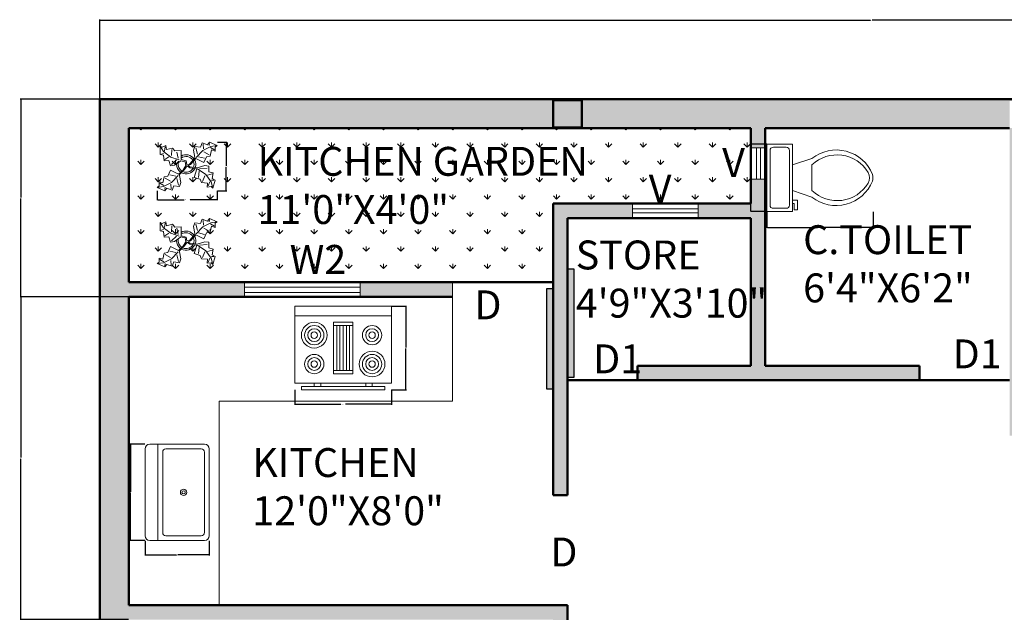
# Model space of a CAD drawing. Units: inches. Extents: x 1099 to 1629, y 1139 to 1548.
# Tile 2 of 3: x 1099 to 1405, y 1364 to 1548. Entities that reach past the tile are written whole.
import ezdxf

# ---------------------------------------------------------------- set-up
doc = ezdxf.new("R2010")
doc.units = ezdxf.units.IN
for name, color, linetype, lineweight in [('A-ANNO-DIMS', 2, 'Continuous', 18), ('A-ANNO-TEXT', 7, 'Continuous', 18), ('A-AREA-IDEN', 7, 'Continuous', 18), ('A-EQPM', 9, 'Continuous', 20), ('A-FLOR-FIXT', 9, 'Continuous', 20), ('A-FURN-FIXD', 2, 'Continuous', 18), ('A-WALL', 1, 'Continuous', 50), ('L-PLNT', 3, 'Continuous', 18), ('L-PLNT-PATT', 3, 'Continuous', 13)]:
    doc.layers.add(name, color=color, linetype=linetype, lineweight=lineweight)
for name, color, linetype, lineweight, true_color in [('A-COLS', 177, 'Continuous', 50, 0x293189), ('A-COLS-PATT', 177, 'Continuous', 13, 0x293189), ('A-DOOR', 30, 'Continuous', 25, 0xf26722), ('A-DOOR-PATT', 30, 'Continuous', 13, 0xf26722), ('A-GLAZ', 177, 'Continuous', 20, 0x293189), ('A-WALL-PATT', 244, 'Continuous', 13, 0x991b1e)]:
    doc.layers.add(name, color=color, linetype=linetype, lineweight=lineweight, true_color=true_color)
doc.styles.get("Standard").update_dxf_attribs({"font": 'arial.ttf'})
doc.dimstyles.get("Standard").update_dxf_attribs({"dimtxt": 0.18, "dimasz": 0.18, "dimexe": 0.18, "dimexo": 0.0625, "dimgap": 0.09, "dimtad": 0, "dimtih": 1, "dimtoh": 1, "dimdec": 4, "dimzin": 0, "dimdsep": 46, "dimtxsty": 'Standard', "dimcen": 0.09, "dimadec": 0, "dimazin": 0, "dimtfac": 1, "dimtdec": 4, "dimtofl": 0, "dimtmove": 0, "dimatfit": 3, "dimfxl": 1, "dimtolj": 1, "dimtzin": 0, "dimarcsym": 0})

# ---------------------------------------------------------------- blocks, each defined once
blk = doc.blocks.new('Toilet - top')
for p, q in [((9.5, -6), (9.5, -2)), ((-10, -8.5), (-8, -8.5)), ((-10, -9.5), (-10, -8.5)), ((-8, -8.5), (-8, -8)), ((-7, -8), (-7, -9.5)), ((-4, -8), (-6, -14)), ((4, -8), (6, -14)), ((-7, -9.5), (-10, -9.5)), ((4, -14), (-4, -14))]:
    blk.add_line(p, q)
blk.add_lwpolyline([(10.5, -8), (10.5, 0), (-10.5, 0), (-10.5, -8)], close=True)
for points in [[(-9.5, -2), (-9.5, -6)], [(8.5, -1), (-8.5, -1)], [(-8.5, -7), (8.5, -7)]]:
    blk.add_lwpolyline(points)
for centre, radius, start, end in [((-8.62, -1.88), 0.884, 81.8699, 188.1301), ((8.62, -1.88), 0.884, 351.8699, 98.1301), ((-8.62, -6.12), 0.884, 171.8699, 278.1301), ((8.62, -6.12), 0.884, 261.8699, 8.1301), ((3.52, -21.58), 12.17, 141.4691, 247.9714), ((4.2, -21.82), 11.33, 136.3677, 238.9468), ((-3.52, -21.58), 12.17, 292.0284, 38.5307), ((-4.2, -21.82), 11.33, 301.053, 43.6321), ((0, -27.88), 4, 245.7318, 294.2682), ((0, -29), 4, 254.8605, 285.1395)]:
    blk.add_arc(centre, radius, start, end)
blk = doc.blocks.new('Range-Oven - 30 in top')
for p, q in [((0, -3), (30, -3)), ((12, -6), (18, -6)), ((13, -20), (13, -6)), ((14, -6), (14, -20)), ((15, -20), (15, -6)), ((16, -6), (16, -20)), ((17, -20), (17, -6)), ((18, -20), (12, -20)), ((6, -24), (6, -25)), ((8, -25), (8, -24)), ((22, -25), (22, -24)), ((24, -24), (24, -25))]:
    blk.add_line(p, q)
for points in [[(0, -24), (0, 0), (30, 0), (30, -24)], [(12, -21), (12, -5), (18, -5), (18, -21)], [(2, -26), (2, -25), (28, -25), (28, -26)]]:
    blk.add_lwpolyline(points, close=True)
for centre, radius in [((6, -9), 4), ((6, -9), 3), ((24, -9), 3), ((6, -9), 2), ((6, -9), 1), ((24, -9), 2), ((24, -9), 1), ((6, -18), 3), ((24, -18), 4), ((24, -18), 3), ((6, -18), 2), ((6, -18), 1), ((24, -18), 2), ((24, -18), 1)]:
    blk.add_circle(centre, radius)
blk = doc.blocks.new('Sink-single - 30 in top')
blk.add_line((-15, -3.999996), (15, -3.999996))
for points in [[(-13.5, 0), (13.5, 0)], [(-15, -18.499996), (-15, -1.5)], [(15, -1.5), (15, -18.499996)], [(-12.5, -5.499996), (12.5, -5.499996)], [(-13.5, -17.499996), (-13.5, -6.499996)], [(13.5, -6.499996), (13.5, -17.499996)], [(13.5, -19.999996), (-13.5, -19.999996)], [(12.5, -18.499996), (-12.5, -18.499996)]]:
    blk.add_lwpolyline(points)
for radius in [1, 0.5]:
    blk.add_circle((0, -11.999996), radius)
for centre, radius, start, end in [((-13.5, -1.5), 1.5, 90, 180), ((13.5, -1.5), 1.5, 0, 90), ((-12.5, -6.499996), 1, 90, 180), ((12.5, -6.499996), 1, 0, 90), ((-12.5, -17.499996), 1, 180, 270), ((12.5, -17.499996), 1, 270, 0), ((-13.5, -18.499996), 1.5, 180, 270), ((13.5, -18.499996), 1.5, 270, 0)]:
    blk.add_arc(centre, radius, start, end)
blk = doc.blocks.new('Plant - Rubber or Philodendron')
for p, q in [((8.8871, 10.7908), (9.9809, 13.4933)), ((9.9809, 13.4933), (13.3837, 12.301)), ((10.5828, 12.6946), (10.8893, 9.7953)), ((13.3837, 12.301), (14.68, 13.9039)), ((14.5816, 13.2037), (14.3848, 11.8033)), ((14.68, 13.9039), (19.3848, 11.8146)), ((-16.2005, 11.4774), (-13.9899, 8.1064)), ((-16.2005, 11.4774), (-14.8639, 10.7964)), ((-16.0159, 6.3329), (-16.2005, 11.4774)), ((-14.0069, 5.8704), (-16.0159, 6.3329)), ((-15.3434, 6.5514), (-13.9984, 6.9884)), ((-14.8639, 10.7964), (-12.6195, 11.8975)), ((-13.9899, 8.1064), (-9.5434, 4.7185)), ((-13.3174, 8.325), (-13.0735, 11.0065)), ((-12.6195, 11.8975), (-12.1909, 9.4345)), ((-12.1909, 9.4345), (-8.3829, 10.3)), ((-8.8369, 9.409), (-9.0894, 5.6095)), ((-8.3829, 10.3), (-7.0549, 8.501)), ((-7.0549, 8.501), (-3.0284, 8.6941)), ((-4.8529, 4.012), (-5.7184, 7.82)), ((-3.0284, 8.6941), (-3.0709, 3.1041)), ((4.6914, 8.8812), (5.3859, 11.2828)), ((4.6914, 8.8812), (5.5014, 4.4831)), ((5.3859, 11.2828), (8.8871, 10.7908)), ((5.9878, 10.4842), (7.1971, 6.3869)), ((10.3916, 8.7942), (6.2847, 4.4028)), ((15.3859, 11.3055), (10.3916, 8.7942)), ((14.2977, 6.1031), (10.9934, 7.9956)), ((15.7909, 9.1065), (14.8995, 5.3044)), ((15.2875, 10.6053), (17.5907, 9.2105)), ((19.3848, 11.8146), (15.3859, 11.3055)), ((18.1925, 8.4119), (15.7909, 9.1065)), ((19.3848, 11.8146), (18.1868, 10.9119)), ((18.1868, 10.9119), (18.1925, 8.4119)), ((-13.5868, 2.2894), (-14.0069, 5.8704)), ((-10.6784, 2.491), (-13.5868, 2.2894)), ((-13.1329, 3.1804), (-10.6614, 4.727)), ((-9.5858, -0.8715), (-10.6784, 2.491)), ((-9.5434, 4.7185), (-4.1917, 2.9888)), ((-9.1318, 0.0195), (-5.9793, 2.9025)), ((-7.1228, -0.443), (-3.5248, 2.2131)), ((-3.5248, 2.2131), (-3.3011, 2.4355)), ((-3.3011, 2.4355), (-0.5306, 1.7947)), ((-3.0709, 3.1041), (0.0797, 2.3163)), ((-0.5306, 1.7947), (-0.2255, -0.5527)), ((-0.5306, 1.7947), (-0.5306, 1.7947)), ((0.0797, 2.3163), (0.4866, -0.031)), ((0.4866, -0.031), (2.1141, 0.2298)), ((2.1141, 0.2298), (5.4346, 3.9146)), ((6.1032, 3.6844), (2.8262, -0.031)), ((5.4346, 3.9146), (5.5014, 4.4831)), ((11.1089, 1.1958), (6.1032, 3.6844)), ((7.7005, 4.8881), (11.5025, 3.9967)), ((12.7005, 4.8994), (11.1089, 1.1958)), ((14.8995, 5.3044), (12.7005, 4.8994)), ((-11.3237, -7.2629), (-9.7321, -3.5593)), ((-9.7321, -3.5593), (-4.7264, -6.0479)), ((-7.1228, -0.443), (-9.5858, -0.8715)), ((-2.019, -3.6148), (-4.7264, -6.0479)), ((-4.0579, -6.2781), (-0.9375, -3.1608)), ((-2.019, -3.6148), (-0.2255, -0.5527)), ((-0.9375, -3.1608), (0.5883, -0.8135)), ((0.5883, -0.8135), (2.2447, -2.0916)), ((2.8262, -0.031), (1.3003, -0.5527)), ((1.3003, -0.5527), (2.4193, -1.4655)), ((2.2447, -2.0916), (6.7108, -2.6626)), ((2.4193, -1.4655), (6.895, -2.1175)), ((4.943, -7.9659), (6.7108, -2.6626)), ((11.6605, -0.5413), (6.895, -2.1175)), ((12.3677, -6.1981), (7.219, -2.6772)), ((8.125, -4.0768), (7.7715, -7.9659)), ((8.3544, -2.7453), (13.1973, -2.1704)), ((11.6605, -0.5413), (14.1354, -0.8948)), ((16.2567, -5.8446), (13.4283, -6.5517)), ((14.1354, -0.8948), (14.1354, -4.4304)), ((14.1354, -4.4304), (16.9638, -5.1375)), ((16.9638, -5.1375), (16.2567, -8.673)), ((-16.8157, -10.7754), (-14.4141, -11.4699)), ((-16.8101, -13.2754), (-16.8157, -10.7754)), ((-13.9107, -12.9688), (-16.2139, -11.574)), ((-14.4141, -11.4699), (-13.5228, -7.6679)), ((-14.0091, -13.669), (-9.0148, -11.1577)), ((-13.5228, -7.6679), (-11.3237, -7.2629)), ((-12.921, -8.4665), (-9.6166, -10.359)), ((-6.3237, -7.2516), (-10.1257, -6.3602)), ((-9.206, -15.0581), (-9.5126, -12.1588)), ((-9.0148, -11.1577), (-4.9047, -6.8122)), ((-4.611, -12.8477), (-5.8203, -8.7504)), ((-4.1246, -6.8466), (-4.0579, -6.2781)), ((-3.3146, -11.2447), (-4.1246, -6.8466)), ((-3.3146, -11.2447), (-4.0092, -13.6463)), ((8.8321, -9.0266), (4.943, -7.9659)), ((9.5392, -11.1479), (8.8321, -9.0266)), ((13.4283, -11.5015), (9.5392, -11.1479)), ((10.2463, -10.4408), (11.6605, -6.9053)), ((15.5496, -10.7943), (12.3677, -6.1981)), ((13.0748, -13.9763), (13.4283, -11.5015)), ((14.8425, -10.7943), (13.7819, -13.2692)), ((16.6103, -14.6834), (15.5496, -10.7943)), ((17.3174, -9.7337), (15.9032, -9.7337)), ((16.2567, -8.673), (18.0245, -9.7337)), ((18.0245, -9.7337), (16.6103, -14.6834)), ((-18.008, -14.1781), (-16.8101, -13.2754)), ((-18.008, -14.1781), (-14.0091, -13.669)), ((-13.3032, -16.2674), (-18.008, -14.1781)), ((-12.0069, -14.6645), (-13.3032, -16.2674)), ((-13.2048, -15.5672), (-13.008, -14.1668)), ((-8.6042, -15.8568), (-12.0069, -14.6645)), ((-7.5103, -13.1543), (-8.6042, -15.8568)), ((-4.0092, -13.6463), (-7.5103, -13.1543)), ((15.5496, -13.6228), (13.0748, -13.9763)), ((16.6103, -14.6834), (15.5496, -13.6228))]:
    blk.add_line(p, q)
for centre, radius, start, end in [((0, 0), 6.1275, 34.37569, 120.1028), ((0.0308, 0.1664), 6, 178.6147, 235.1169), ((0.0308, 0.1664), 5, 168.1647, 238.6725), ((-0.0601, -0.2075), 5.2461, 33.82192, 124.9414), ((-0.2664, 0.1682), 5.2775, 338.4094, 20.03007), ((-0.098, 0.1364), 6.1288, 341.2017, 26.09184), ((-0.0234, 0.3825), 6.1492, 242.5812, 331.2714), ((-0.1102, 0.4886), 5.2883, 247.3711, 327.472)]:
    blk.add_arc(centre, radius, start, end)
blk = doc.blocks.new('*D11')
at = {"layer": 'A-ANNO-DIMS', "color": 0, "lineweight": -2, "transparency": 16777216}
for p, q in [((1331.62, 1488.62), (1331.62, 1483.55)), ((1364.67, 1488.62), (1364.67, 1483.55)), ((1331.8, 1483.73), (1347.37, 1483.73)), ((1364.49, 1483.73), (1348.92, 1483.73))]:
    blk.add_line(p, q, dxfattribs=at)
at = {"layer": 'A-ANNO-DIMS', "color": 0, "lineweight": 100, "transparency": 16777216}
for points in [[(1331.8, 1483.76), (1331.8, 1483.7), (1331.62, 1483.73)], [(1364.49, 1483.76), (1364.49, 1483.7), (1364.67, 1483.73)]]:
    blk.add_solid(points, dxfattribs=at)
at = {"layer": 'Defpoints', "color": 0, "lineweight": 100, "transparency": 16777216}
for p in [(1331.62, 1488.69), (1364.67, 1488.69), (1331.62, 1483.73)]:
    blk.add_point(p, dxfattribs=at)
at = {"layer": 'A-ANNO-DIMS', "color": 0, "transparency": 16777216, "insert": (1348.14, 1483.73), "char_height": 0.18, "attachment_point": 5}
blk.add_mtext('\\A1;WC 33 TYP.', dxfattribs=at)
blk = doc.blocks.new('*D12')
at = {"layer": 'A-ANNO-DIMS', "color": 0, "lineweight": -2, "transparency": 16777216}
for p, q in [((1331.56, 1509.69), (1326.48, 1509.69)), ((1326.66, 1509.51), (1326.66, 1499.37)), ((1326.66, 1488.87), (1326.66, 1499)), ((1331.56, 1488.69), (1326.48, 1488.69))]:
    blk.add_line(p, q, dxfattribs=at)
at = {"layer": 'A-ANNO-DIMS', "color": 0, "lineweight": 100, "transparency": 16777216}
for points in [[(1326.63, 1509.51), (1326.69, 1509.51), (1326.66, 1509.69)], [(1326.63, 1488.87), (1326.69, 1488.87), (1326.66, 1488.69)]]:
    blk.add_solid(points, dxfattribs=at)
at = {"layer": 'Defpoints', "color": 0, "lineweight": 100, "transparency": 16777216}
for p in [(1326.66, 1509.69), (1331.62, 1509.69), (1331.62, 1488.69)]:
    blk.add_point(p, dxfattribs=at)
at = {"layer": 'A-ANNO-DIMS', "color": 0, "transparency": 16777216, "insert": (1326.66, 1499.19), "char_height": 0.18, "attachment_point": 5}
blk.add_mtext('\\A1;21 TYP.', dxfattribs=at)
blk = doc.blocks.new('*D15')
at = {"layer": 'A-ANNO-DIMS', "color": 0, "lineweight": -2, "transparency": 16777216}
for p, q in [((1184.82, 1433.12), (1184.82, 1428.5)), ((1214.82, 1433.12), (1214.82, 1428.5)), ((1185, 1428.68), (1199.12, 1428.68)), ((1214.64, 1428.68), (1200.51, 1428.68))]:
    blk.add_line(p, q, dxfattribs=at)
at = {"layer": 'A-ANNO-DIMS', "color": 0, "lineweight": 100, "transparency": 16777216}
for points in [[(1185, 1428.71), (1185, 1428.65), (1184.82, 1428.68)], [(1214.64, 1428.71), (1214.64, 1428.65), (1214.82, 1428.68)]]:
    blk.add_solid(points, dxfattribs=at)
at = {"layer": 'Defpoints', "color": 0, "lineweight": 100, "transparency": 16777216}
for p in [(1184.82, 1433.18), (1214.82, 1433.18), (1214.82, 1428.68)]:
    blk.add_point(p, dxfattribs=at)
at = {"layer": 'A-ANNO-DIMS', "color": 0, "transparency": 16777216, "insert": (1199.82, 1428.68), "char_height": 0.18, "attachment_point": 5}
blk.add_mtext('\\A1;RANGE 30', dxfattribs=at)
blk = doc.blocks.new('*D16')
at = {"layer": 'A-ANNO-DIMS', "color": 0, "lineweight": -2, "transparency": 16777216}
for p, q in [((1214.88, 1459.18), (1219.5, 1459.18)), ((1219.32, 1459), (1219.32, 1446.36)), ((1219.32, 1433.36), (1219.32, 1446)), ((1214.88, 1433.18), (1219.5, 1433.18))]:
    blk.add_line(p, q, dxfattribs=at)
at = {"layer": 'A-ANNO-DIMS', "color": 0, "lineweight": 100, "transparency": 16777216}
for points in [[(1219.29, 1459), (1219.35, 1459), (1219.32, 1459.18)], [(1219.29, 1433.36), (1219.35, 1433.36), (1219.32, 1433.18)]]:
    blk.add_solid(points, dxfattribs=at)
at = {"layer": 'Defpoints', "color": 0, "lineweight": 100, "transparency": 16777216}
for p in [(1214.82, 1459.18), (1219.32, 1459.18), (1214.82, 1433.18)]:
    blk.add_point(p, dxfattribs=at)
at = {"layer": 'A-ANNO-DIMS', "color": 0, "transparency": 16777216, "insert": (1219.32, 1446.18), "char_height": 0.18, "attachment_point": 5}
blk.add_mtext('\\A1;26', dxfattribs=at)
blk = doc.blocks.new('*D17')
at = {"layer": 'A-ANNO-DIMS', "color": 0, "lineweight": -2, "transparency": 16777216}
for p, q in [((1138.11, 1416.24), (1133.5, 1416.24)), ((1133.68, 1416.06), (1133.68, 1401.42)), ((1133.68, 1386.42), (1133.68, 1401.06)), ((1138.11, 1386.24), (1133.5, 1386.24))]:
    blk.add_line(p, q, dxfattribs=at)
at = {"layer": 'A-ANNO-DIMS', "color": 0, "lineweight": 100, "transparency": 16777216}
for points in [[(1133.65, 1416.06), (1133.71, 1416.06), (1133.68, 1416.24)], [(1133.65, 1386.42), (1133.71, 1386.42), (1133.68, 1386.24)]]:
    blk.add_solid(points, dxfattribs=at)
at = {"layer": 'Defpoints', "color": 0, "lineweight": 100, "transparency": 16777216}
for p in [(1133.68, 1416.24), (1138.18, 1416.24), (1138.18, 1386.24)]:
    blk.add_point(p, dxfattribs=at)
at = {"layer": 'A-ANNO-DIMS', "color": 0, "transparency": 16777216, "insert": (1133.68, 1401.24), "char_height": 0.18, "attachment_point": 5}
blk.add_mtext('\\A1;SINK 30', dxfattribs=at)
blk = doc.blocks.new('*D18')
at = {"layer": 'A-ANNO-DIMS', "color": 0, "lineweight": -2, "transparency": 16777216}
for p, q in [((1138.18, 1386.18), (1138.18, 1381.56)), ((1158.18, 1386.18), (1158.18, 1381.56)), ((1138.36, 1381.74), (1147.96, 1381.74)), ((1158, 1381.74), (1148.4, 1381.74))]:
    blk.add_line(p, q, dxfattribs=at)
at = {"layer": 'A-ANNO-DIMS', "color": 0, "lineweight": 100, "transparency": 16777216}
for points in [[(1138.36, 1381.77), (1138.36, 1381.71), (1138.18, 1381.74)], [(1158, 1381.77), (1158, 1381.71), (1158.18, 1381.74)]]:
    blk.add_solid(points, dxfattribs=at)
at = {"layer": 'Defpoints', "color": 0, "lineweight": 100, "transparency": 16777216}
for p in [(1138.18, 1386.24), (1158.18, 1386.24), (1138.18, 1381.74)]:
    blk.add_point(p, dxfattribs=at)
at = {"layer": 'A-ANNO-DIMS', "color": 0, "transparency": 16777216, "insert": (1148.18, 1381.74), "char_height": 0.18, "attachment_point": 5}
blk.add_mtext('\\A1;20', dxfattribs=at)
blk = doc.blocks.new('*D23')
at = {"layer": 'A-ANNO-DIMS', "color": 0, "lineweight": -2, "transparency": 16777216}
for p, q in [((1141.94, 1495.09), (1141.94, 1492.17)), ((1160.64, 1495.09), (1160.64, 1492.17)), ((1142.12, 1492.35), (1150.32, 1492.35)), ((1160.46, 1492.35), (1152.25, 1492.35))]:
    blk.add_line(p, q, dxfattribs=at)
at = {"layer": 'A-ANNO-DIMS', "color": 0, "lineweight": 100, "transparency": 16777216}
for points in [[(1142.12, 1492.38), (1142.12, 1492.32), (1141.94, 1492.35)], [(1160.46, 1492.38), (1160.46, 1492.32), (1160.64, 1492.35)]]:
    blk.add_solid(points, dxfattribs=at)
at = {"layer": 'Defpoints', "color": 0, "lineweight": 100, "transparency": 16777216}
for p in [(1141.94, 1495.16), (1160.64, 1495.16), (1160.64, 1492.35)]:
    blk.add_point(p, dxfattribs=at)
at = {"layer": 'A-ANNO-DIMS', "color": 0, "transparency": 16777216, "insert": (1151.29, 1492.35), "char_height": 0.18, "attachment_point": 5}
blk.add_mtext('\\A1;PLANT 19 TYP.', dxfattribs=at)
blk = doc.blocks.new('*D24')
at = {"layer": 'A-ANNO-DIMS', "color": 0, "lineweight": -2, "transparency": 16777216}
for p, q in [((1160.7, 1510.24), (1163.62, 1510.24)), ((1163.44, 1510.06), (1163.44, 1502.88)), ((1163.44, 1495.34), (1163.44, 1502.52)), ((1160.7, 1495.16), (1163.62, 1495.16))]:
    blk.add_line(p, q, dxfattribs=at)
at = {"layer": 'A-ANNO-DIMS', "color": 0, "lineweight": 100, "transparency": 16777216}
for points in [[(1163.41, 1510.06), (1163.47, 1510.06), (1163.44, 1510.24)], [(1163.41, 1495.34), (1163.47, 1495.34), (1163.44, 1495.16)]]:
    blk.add_solid(points, dxfattribs=at)
at = {"layer": 'Defpoints', "color": 0, "lineweight": 100, "transparency": 16777216}
for p in [(1160.64, 1510.24), (1163.44, 1510.24), (1160.64, 1495.16)]:
    blk.add_point(p, dxfattribs=at)
at = {"layer": 'A-ANNO-DIMS', "color": 0, "transparency": 16777216, "insert": (1163.44, 1502.7), "char_height": 0.18, "attachment_point": 5}
blk.add_mtext('\\A1;15 TYP.', dxfattribs=at)
blk = doc.blocks.new('*D25')
at = {"layer": 'A-ANNO-DIMS', "color": 0, "lineweight": -2, "transparency": 16777216}
for p, q in [((1124.1, 1523.69), (1124.1, 1548.41)), ((1124.28, 1548.23), (1363.81, 1548.23)), ((1603.92, 1548.23), (1364.39, 1548.23)), ((1604.1, 1523.69), (1604.1, 1548.41))]:
    blk.add_line(p, q, dxfattribs=at)
at = {"layer": 'A-ANNO-DIMS', "color": 0, "lineweight": 100, "transparency": 16777216}
for points in [[(1124.28, 1548.26), (1124.28, 1548.2), (1124.1, 1548.23)], [(1603.92, 1548.26), (1603.92, 1548.2), (1604.1, 1548.23)]]:
    blk.add_solid(points, dxfattribs=at)
at = {"layer": 'Defpoints', "color": 0, "lineweight": 100, "transparency": 16777216}
for p in [(1604.1, 1548.23), (1124.1, 1523.63), (1604.1, 1523.63)]:
    blk.add_point(p, dxfattribs=at)
at = {"layer": 'A-ANNO-DIMS', "color": 0, "transparency": 16777216, "insert": (1364.1, 1548.23), "char_height": 0.18, "attachment_point": 5}
blk.add_mtext('\\A1;480', dxfattribs=at)
blk = doc.blocks.new('*D36')
at = {"layer": 'A-ANNO-DIMS', "color": 0, "lineweight": -2, "transparency": 16777216}
for p, q in [((1133.04, 1462.13), (1099.32, 1462.13)), ((1099.5, 1461.95), (1099.5, 1412.06)), ((1099.5, 1361.81), (1099.5, 1411.7)), ((1133.04, 1361.63), (1099.32, 1361.63))]:
    blk.add_line(p, q, dxfattribs=at)
at = {"layer": 'A-ANNO-DIMS', "color": 0, "lineweight": 100, "transparency": 16777216}
for points in [[(1099.47, 1461.95), (1099.53, 1461.95), (1099.5, 1462.13)], [(1099.47, 1361.81), (1099.53, 1361.81), (1099.5, 1361.63)]]:
    blk.add_solid(points, dxfattribs=at)
at = {"layer": 'Defpoints', "color": 0, "lineweight": 100, "transparency": 16777216}
for p in [(1099.5, 1462.13), (1133.1, 1462.13), (1133.1, 1361.63)]:
    blk.add_point(p, dxfattribs=at)
at = {"layer": 'A-ANNO-DIMS', "color": 0, "transparency": 16777216, "insert": (1099.5, 1411.88), "char_height": 0.18, "attachment_point": 5}
blk.add_mtext('\\A1;100.5', dxfattribs=at)
blk = doc.blocks.new('*D37')
at = {"layer": 'A-ANNO-DIMS', "color": 0, "lineweight": -2, "transparency": 16777216}
for p, q in [((1124.04, 1523.63), (1099.32, 1523.63)), ((1099.5, 1523.45), (1099.5, 1493.06)), ((1099.5, 1462.31), (1099.5, 1492.7)), ((1133.04, 1462.13), (1099.32, 1462.13))]:
    blk.add_line(p, q, dxfattribs=at)
at = {"layer": 'A-ANNO-DIMS', "color": 0, "lineweight": 100, "transparency": 16777216}
for points in [[(1099.47, 1523.45), (1099.53, 1523.45), (1099.5, 1523.63)], [(1099.47, 1462.31), (1099.53, 1462.31), (1099.5, 1462.13)]]:
    blk.add_solid(points, dxfattribs=at)
at = {"layer": 'Defpoints', "color": 0, "lineweight": 100, "transparency": 16777216}
for p in [(1099.5, 1523.63), (1124.1, 1523.63), (1133.1, 1462.13)]:
    blk.add_point(p, dxfattribs=at)
at = {"layer": 'A-ANNO-DIMS', "color": 0, "transparency": 16777216, "insert": (1099.5, 1492.88), "char_height": 0.18, "attachment_point": 5}
blk.add_mtext('\\A1;61.5', dxfattribs=at)

msp = doc.modelspace()

# ---------------------------------------------------------------- hatches: boundary and pattern name
at = {"layer": 'A-COLS-PATT'}
h = msp.add_hatch(color=256, dxfattribs=at)
h.dxf.hatch_style = 1
h.paths.add_polyline_path([(1265.099, 1514.872), (1274.099, 1514.872), (1274.099, 1523.316), (1265.099, 1523.316)])
at = {"layer": 'A-DOOR-PATT'}
h = msp.add_hatch(color=256, dxfattribs=at)
h.dxf.hatch_style = 1
h.paths.add_polyline_path([(1265.099, 1464.652), (1263.099, 1464.652), (1263.099, 1433.449), (1265.099, 1433.449)])
h.paths.add_polyline_path([(1271.599, 1470.878), (1269.599, 1470.878), (1269.599, 1437.014), (1271.599, 1437.014)])
at = {"layer": 'A-WALL-PATT'}
h = msp.add_hatch(color=256, dxfattribs=at)
h.dxf.hatch_style = 1
h.paths.add_polyline_path([(1407.099, 1523.072), (1416.099, 1523.072), (1416.099, 1514.628), (1595.099, 1514.628), (1595.099, 1523.072), (1604.099, 1523.072), (1604.099, 1523.628), (1124.099, 1523.628), (1124.099, 1172.072), (1133.099, 1172.072), (1133.099, 1361.628), (1265.099, 1361.628), (1265.099, 1301.628), (1269.599, 1301.628), (1269.599, 1366.128), (1133.099, 1366.128), (1133.099, 1462.128), (1169.127, 1462.128), (1169.127, 1466.628), (1133.099, 1466.628), (1133.099, 1514.628), (1265.099, 1514.628), (1265.099, 1514.872), (1265.099, 1523.316), (1274.099, 1523.316), (1274.099, 1514.628), (1326.599, 1514.628), (1326.599, 1508.465), (1331.099, 1508.465), (1331.099, 1514.628), (1407.099, 1514.628)])
h.paths.add_polyline_path([(1604.099, 1514.628), (1595.099, 1514.628), (1595.099, 1384.628), (1595.099, 1380.128), (1595.099, 1323.878), (1535.099, 1323.878), (1535.099, 1321.628), (1595.099, 1321.628), (1595.099, 1172.628), (1539.988, 1172.628), (1539.988, 1163.628), (1594.904, 1163.628), (1594.904, 1172.072), (1604.099, 1172.072)])
h.paths.add_polyline_path([(1461.599, 1380.128), (1530.599, 1380.128), (1530.599, 1363.564), (1535.099, 1363.564), (1535.099, 1380.128), (1535.099, 1384.628), (1416.099, 1384.628), (1416.099, 1380.128), (1457.099, 1380.128), (1457.099, 1326.128), (1457.099, 1321.628), (1504.951, 1321.628), (1504.951, 1326.128), (1461.599, 1326.128)], flags=17)
h.paths.add_polyline_path([(1535.099, 1346.252), (1530.599, 1346.252), (1530.599, 1326.128), (1530.599, 1321.628), (1535.099, 1321.628), (1535.099, 1323.878), (1535.099, 1326.128)], flags=16)
h.paths.add_polyline_path([(1269.599, 1301.628), (1265.099, 1301.628), (1260.599, 1301.628), (1260.599, 1214.628), (1260.599, 1205.628), (1265.099, 1205.628), (1269.599, 1205.628), (1269.599, 1214.628)], flags=17)
h.paths.add_polyline_path([(1411.599, 1262.279), (1451.001, 1262.279), (1451.001, 1266.779), (1411.599, 1266.779), (1411.599, 1342.184), (1407.099, 1342.184), (1407.099, 1214.628), (1386.727, 1214.628), (1386.727, 1205.628), (1407.099, 1205.628), (1407.099, 1163.628), (1491.988, 1163.628), (1491.988, 1172.628), (1411.599, 1172.628)])
h.paths.add_polyline_path([(1315.906, 1214.628), (1300.958, 1214.628), (1300.958, 1205.628), (1315.906, 1205.628)], flags=17)
h = msp.add_hatch(color=256, dxfattribs=at)
h.dxf.hatch_style = 1
h.paths.add_polyline_path([(1233.806, 1466.628), (1205.127, 1466.628), (1205.127, 1462.128), (1233.806, 1462.128)])
h.paths.add_polyline_path([(1269.599, 1486.628), (1289.77, 1486.628), (1289.77, 1491.128), (1269.599, 1491.128), (1265.099, 1491.128), (1265.099, 1400.307), (1269.599, 1400.307)])
h.paths.add_polyline_path([(1379.104, 1440.628), (1331.099, 1440.628), (1331.099, 1498.77), (1326.599, 1498.77), (1326.599, 1491.128), (1310.198, 1491.128), (1310.198, 1486.628), (1326.599, 1486.628), (1326.599, 1440.628), (1291.317, 1440.628), (1291.317, 1436.128), (1379.104, 1436.128)])
h.paths.add_polyline_path([(1416.099, 1514.628), (1407.099, 1514.628), (1407.099, 1418.838), (1411.599, 1418.838), (1438.846, 1418.838), (1438.846, 1423.338), (1416.099, 1423.338)])
at = {"layer": 'L-PLNT-PATT'}
h = msp.add_hatch(dxfattribs=at)
h.set_pattern_fill('GRASS', color=256, scale=0.3)
h.paths.add_polyline_path([(1265.099, 1491.128), (1269.599, 1491.128), (1326.599, 1491.128), (1326.599, 1514.628), (1133.099, 1514.628), (1133.099, 1466.628), (1265.099, 1466.628)])

# ---------------------------------------------------------------- linework, layer by layer
at = {"layer": 'A-COLS'}
msp.add_lwpolyline([(1265.099, 1514.872), (1274.099, 1514.872), (1274.099, 1523.316), (1265.099, 1523.316)], close=True, dxfattribs=at)
at = {"layer": 'A-DOOR'}
for p, q in [((1269.599, 1470.878), (1271.599, 1470.878)), ((1271.599, 1470.878), (1271.599, 1437.014)), ((1265.099, 1464.652), (1263.099, 1464.652)), ((1263.099, 1464.652), (1263.099, 1433.449)), ((1271.599, 1437.014), (1269.599, 1437.014)), ((1263.099, 1433.449), (1265.099, 1433.449))]:
    msp.add_line(p, q, dxfattribs=at)
at = {"layer": 'A-FURN-FIXD'}
for p, q in [((1233.806, 1466.628), (1233.806, 1438.761)), ((1233.806, 1438.761), (1233.806, 1429.661)), ((1161.284, 1429.661), (1161.284, 1366.128)), ((1233.806, 1429.661), (1161.284, 1429.661))]:
    msp.add_line(p, q, dxfattribs=at)
at = {"layer": 'A-GLAZ'}
for p, q in [((1331.099, 1508.465), (1326.599, 1508.465)), ((1328.406, 1508.465), (1328.406, 1498.77)), ((1329.664, 1508.465), (1329.664, 1498.77)), ((1331.099, 1498.77), (1326.599, 1498.77)), ((1289.77, 1491.128), (1289.77, 1486.628)), ((1310.198, 1489.495), (1289.77, 1489.495)), ((1310.198, 1491.128), (1310.198, 1486.628)), ((1310.198, 1488.239), (1289.77, 1488.239)), ((1169.127, 1466.628), (1169.127, 1462.128)), ((1169.127, 1465.16), (1205.127, 1465.16)), ((1205.127, 1466.628), (1205.127, 1462.128)), ((1169.127, 1463.462), (1205.127, 1463.462))]:
    msp.add_line(p, q, dxfattribs=at)
at = {"layer": 'A-WALL'}
for p, q in [((1604.099, 1523.628), (1124.099, 1523.628)), ((1124.099, 1523.628), (1124.099, 1163.628)), ((1133.099, 1514.628), (1133.099, 1466.628)), ((1265.099, 1514.628), (1133.099, 1514.628)), ((1326.599, 1514.628), (1133.099, 1514.628)), ((1326.599, 1514.628), (1326.599, 1491.128)), ((1407.099, 1514.628), (1331.099, 1514.628)), ((1331.099, 1514.628), (1331.099, 1440.628)), ((1265.099, 1491.128), (1265.099, 1400.307)), ((1269.599, 1491.128), (1265.099, 1491.128)), ((1326.599, 1491.128), (1269.599, 1491.128)), ((1326.599, 1486.628), (1269.599, 1486.628)), ((1269.599, 1486.628), (1269.599, 1400.307)), ((1326.599, 1486.628), (1326.599, 1440.628)), ((1265.099, 1466.628), (1133.099, 1466.628)), ((1233.806, 1462.128), (1133.099, 1462.128)), ((1133.099, 1462.128), (1133.099, 1366.128)), ((1326.599, 1440.628), (1291.317, 1440.628)), ((1291.317, 1440.628), (1291.317, 1436.128)), ((1379.104, 1440.628), (1331.099, 1440.628)), ((1379.104, 1440.628), (1379.104, 1436.128)), ((1407.099, 1436.128), (1269.599, 1436.128)), ((1269.599, 1400.307), (1265.099, 1400.307)), ((1269.599, 1366.128), (1133.099, 1366.128)), ((1269.599, 1366.128), (1269.599, 1301.628))]:
    msp.add_line(p, q, dxfattribs=at)

# ---------------------------------------------------------------- block references
at = {"layer": 'A-EQPM'}
msp.add_blockref('Range-Oven - 30 in top', (1184.816, 1459.179), dxfattribs=at)
at = {"layer": 'A-FLOR-FIXT'}
for name, p, rotation in [('Toilet - top', (1331.62, 1499.185), 89.99999999999953), ('Sink-single - 30 in top', (1138.177, 1401.239), 90)]:
    msp.add_blockref(name, p, dxfattribs=dict(at, rotation=rotation))
at = {"layer": 'L-PLNT', "xscale": 0.5, "yscale": 0.5}
for p in [(1150.943, 1503.29), (1150.943, 1479.542)]:
    msp.add_blockref('Plant - Rubber or Philodendron', p, dxfattribs=at)

# ---------------------------------------------------------------- texts
at = {"layer": 'A-ANNO-TEXT', "char_height": 9, "attachment_point": 1}
for s, insert in [('V', (1317.714, 1508.43)), ('V', (1294.873, 1500.128)), ('W2', (1183.174, 1478.263)), ('D', (1240.626, 1464.109)), ('D1', (1389.369, 1448.849)), ('D1', (1277.564, 1447.298)), ('D', (1264.238, 1387.154))]:
    msp.add_mtext_dynamic_manual_height_columns(s, width=16.11456, gutter_width=12.5, heights=[0], dxfattribs=dict(at, insert=insert))
at = {"layer": 'A-AREA-IDEN', "char_height": 9, "attachment_point": 1}
for s, width, insert in [('KITCHEN GARDEN\\P11\'0"X4\'0"', 121.65143, (1173.174, 1508.795)), ('C.TOILET\\P6\'4"X6\'2"', 79.89808, (1342.884, 1484.398)), ('STORE\\P4\'9"X3\'10"', 79.89808, (1272.149, 1479.645)), ('KITCHEN\\P12\'0"X8\'0"', 79.89808, (1171.552, 1415.009))]:
    msp.add_mtext_dynamic_manual_height_columns(s, width=width, gutter_width=12.5, heights=[0], dxfattribs=dict(at, insert=insert))

# ---------------------------------------------------------------- dimensions: what is measured, and where the dimension line sits
at = {"layer": 'A-ANNO-DIMS'}
dim = msp.add_linear_dim(base=(1604.099, 1548.228), p1=(1124.099, 1523.628), p2=(1604.099, 1523.628), dimstyle='Standard', override={"dimdec": 0, "dimlfac": 1, "dimrnd": 0, "dimzin": 0, "dimdsep": 46, "dimlunit": 2}, dxfattribs=at)
dim.commit()
dim.dimension.update_dxf_attribs({"geometry": '*D25', "text_midpoint": (1364.099, 1548.228)})
for base, p1, p2, angle, override, picture, middle in [((1099.499, 1523.628), (1133.099, 1462.128), (1124.099, 1523.628), 90, {"dimdec": 1, "dimlfac": 1, "dimrnd": 0, "dimzin": 0, "dimdsep": 46, "dimlunit": 2}, '*D37', (1099.499, 1492.878)), ((1099.499, 1462.128), (1133.099, 1361.628), (1133.099, 1462.128), 90, {"dimdec": 1, "dimlfac": 1, "dimrnd": 0, "dimzin": 0, "dimdsep": 46, "dimlunit": 2}, '*D36', (1099.499, 1411.878)), ((1219.316, 1459.179), (1214.816, 1433.179), (1214.816, 1459.179), 90, {"dimdec": 0, "dimlfac": 1, "dimrnd": 0, "dimzin": 0, "dimdsep": 46, "dimlunit": 2}, '*D16', (1219.316, 1446.179)), ((1138.177, 1381.739), (1158.177, 1386.239), (1138.177, 1386.239), 180, {"dimdec": 0, "dimlfac": 1, "dimrnd": 0, "dimzin": 0, "dimdsep": 46, "dimlunit": 2}, '*D18', (1148.177, 1381.739))]:
    dim = msp.add_linear_dim(base=base, p1=p1, p2=p2, angle=angle, dimstyle='Standard', override=override, dxfattribs=at)
    dim.commit()
    dim.dimension.update_dxf_attribs({"geometry": picture, "text_midpoint": middle})
for base, p1, p2, angle, text, picture, middle in [((1163.44, 1510.242), (1160.635, 1495.156), (1160.635, 1510.242), 90, '<> TYP.', '*D24', (1163.44, 1502.699)), ((1326.663, 1509.685), (1331.62, 1488.685), (1331.62, 1509.685), 90, '<> TYP.', '*D12', (1326.663, 1499.185)), ((1331.62, 1483.728), (1364.666, 1488.685), (1331.62, 1488.685), 180, 'WC <> TYP.', '*D11', (1348.143, 1483.728)), ((1133.677, 1416.239), (1138.177, 1386.239), (1138.177, 1416.239), 90, 'SINK <>', '*D17', (1133.677, 1401.239))]:
    dim = msp.add_linear_dim(base=base, p1=p1, p2=p2, angle=angle, text=text, dimstyle='Standard', override={"dimdec": 0, "dimlfac": 1, "dimrnd": 0, "dimzin": 0, "dimdsep": 46, "dimlunit": 2}, dxfattribs=at)
    dim.commit()
    dim.dimension.update_dxf_attribs({"geometry": picture, "text_midpoint": middle})
for base, p1, p2, text, picture, middle in [((1160.635, 1492.352), (1141.939, 1495.156), (1160.635, 1495.156), 'PLANT <> TYP.', '*D23', (1151.287, 1492.352)), ((1214.816, 1428.679), (1184.816, 1433.179), (1214.816, 1433.179), 'RANGE <>', '*D15', (1199.816, 1428.679))]:
    dim = msp.add_linear_dim(base=base, p1=p1, p2=p2, text=text, dimstyle='Standard', override={"dimdec": 0, "dimlfac": 1, "dimrnd": 0, "dimzin": 0, "dimdsep": 46, "dimlunit": 2}, dxfattribs=at)
    dim.commit()
    dim.dimension.update_dxf_attribs({"geometry": picture, "text_midpoint": middle})

doc.saveas('drawing.dxf')
